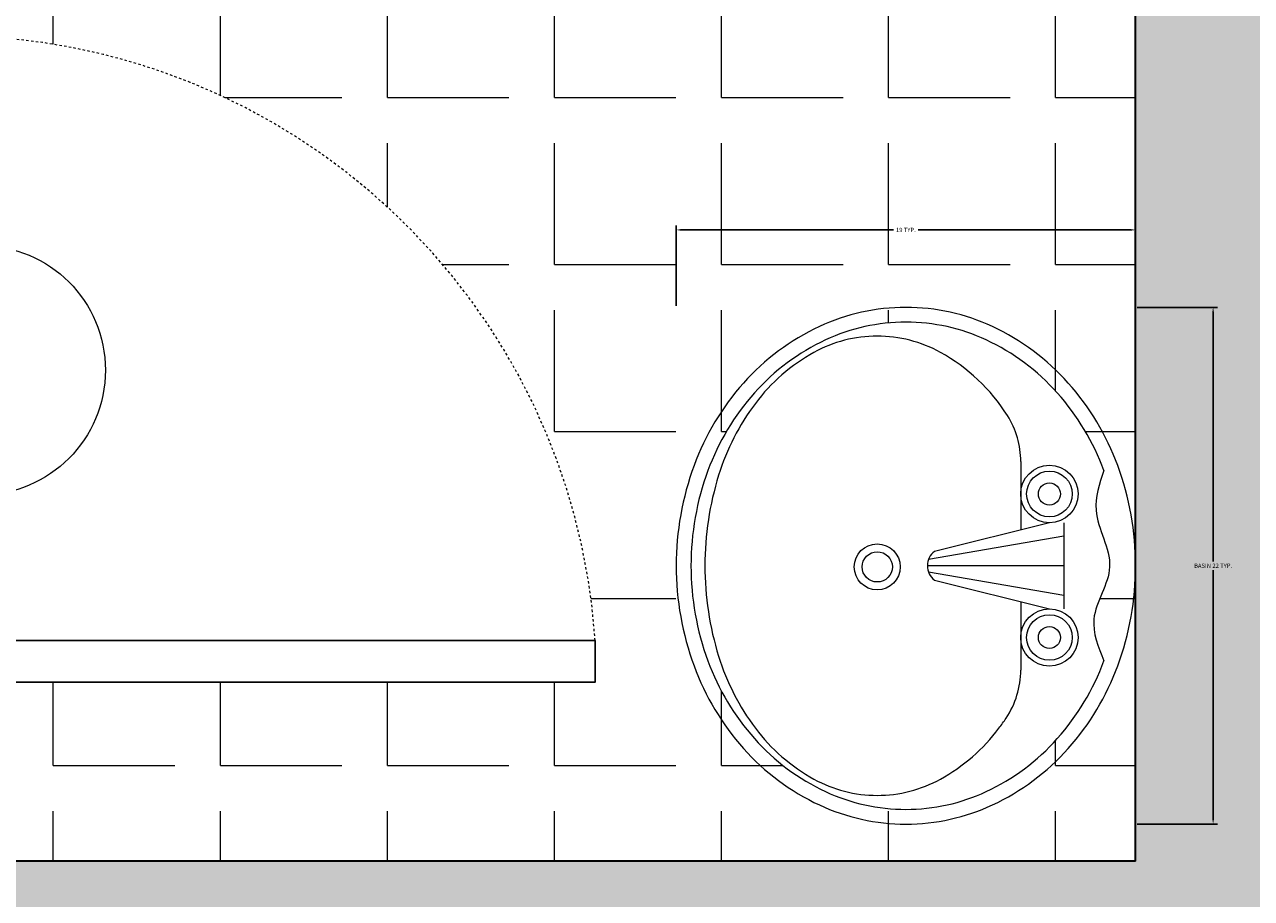
# Model space of a CAD drawing. Units: inches. Extents: x 2701 to 6846, y 811 to 2447.
# Tile 17 of 20: x 2926 to 2977, y 1370 to 1407. Entities that reach past the tile are written whole.
import ezdxf

# ---------------------------------------------------------------- set-up
doc = ezdxf.new("R2010")
doc.units = ezdxf.units.IN
doc.linetypes.add('HIDDEN4', pattern=[0.09375, 0.0625, -0.03125])
for name, color, linetype, lineweight in [('A-ANNO-DIMS', 2, 'Continuous', 18), ('A-ANNO-IDEN', 7, 'Continuous', 13), ('A-DOOR', 4, 'Continuous', 25), ('A-DOOR-SWNG', 4, 'HIDDEN4', 13), ('A-FLOR-FIXT', 7, 'Continuous', 18), ('A-FLOR-PATT', 252, 'Continuous', 13), ('A-WALL', 7, 'Continuous', 35)]:
    doc.layers.add(name, color=color, linetype=linetype, lineweight=lineweight)
doc.layers.add('A-WALL-PATT', color=18, linetype='Continuous', lineweight=13, true_color=0x000000)
doc.styles.get("Standard").update_dxf_attribs({"font": 'arial.ttf'})
doc.dimstyles.get("Standard").update_dxf_attribs({"dimtxt": 0.18, "dimasz": 0.18, "dimexe": 0.18, "dimexo": 0.0625, "dimgap": 0.09, "dimtad": 0, "dimtih": 1, "dimtoh": 1, "dimdec": 4, "dimzin": 0, "dimdsep": 46, "dimtxsty": 'Standard', "dimcen": 0.09, "dimadec": 0, "dimazin": 0, "dimtfac": 1, "dimtdec": 4, "dimtofl": 0, "dimtmove": 0, "dimatfit": 3, "dimfxl": 1, "dimtolj": 1, "dimtzin": 0, "dimarcsym": 0})

# ---------------------------------------------------------------- blocks, each defined once
blk = doc.blocks.new('A$C62EA08CE')
at = {"linetype": 'ByBlock'}
for p, q in [((0.2190750854661019, 0.3943350335612194), (0.306705085467911, 0.3943350335612194)), ((0.2328389724007138, 0.3943350335612194), (0.256592247476874, 0.2566437564746593)), ((0.2628900854706444, 0.3943350335612194), (0.2628900854706444, 0.2555161210839287)), ((0.2933077018988115, 0.3943350335612194), (0.2695802776597702, 0.256794098582759)), ((0.2190750854661019, 0.3797300335645559), (0.2482850854667049, 0.2628900335621438)), ((0.2774950854673079, 0.2628900335621438), (0.306705085467911, 0.3797300335645559)), ((0.1569030901755468, 0.3505200335639529), (0.2263775854680716, 0.3505200335639529)), ((0.2994025854659412, 0.3505200335639529), (0.3690778702966782, 0.3505200335639529))]:
    blk.add_line(p, q, dxfattribs=at)
for centre, radius in [((0.1898650854727748, 0.3797300335645559), 0.02921), ((0.1898650854727748, 0.3797300335645559), 0.02321), ((0.335915085468514, 0.3797300335645559), 0.02921), ((0.335915085468514, 0.3797300335645559), 0.02321), ((0.1898650854727748, 0.3797300335645559), 0.01121), ((0.335915085468514, 0.3797300335645559), 0.01121), ((0.2640384579517558, 0.2045255693010404), 0.023368), ((0.2640384579517558, 0.2045255693010404), 0.015368)]:
    blk.add_circle(centre, radius, dxfattribs=at)
for centre, radius, start, end in [((0.2628901093212335, 0.172201390065311), 0.2951586434963838, 90.00000458569829, 110.2131769401282), ((0.2628900616127794, 0.172201390065311), 0.2951586434963838, 69.78682305987175, 89.9999954143017), ((0.2518357941607974, 0.202225176646607), 0.2631644933429036, 110.2132031902237, 131.6335499305747), ((0.2739443767732155, 0.202225176646607), 0.2631644933429035, 48.36645006942531, 69.78679680977629), ((0.2518357941607974, 0.202225176646607), 0.2481644933429036, 110.2132031902237, 131.6335499305747), ((0.2739443767732155, 0.202225176646607), 0.2481644933429035, 48.36645006942531, 69.78679680977629), ((0.2348020259832992, 0.2213881285715615), 0.2375253048786466, 131.6335451873388, 155.0149376704166), ((0.2348020259832992, 0.2213881285715615), 0.2225253048786466, 131.6335451873388, 155.0149376704166), ((0.2909781449579896, 0.2213881285715615), 0.2225253048786464, 24.98506232958336, 48.36645481266113), ((0.2909781449579896, 0.2213881285715615), 0.2375253048786464, 24.98506232958336, 48.36645481266113), ((0.1569030901755468, 0.2628900335621438), 0.08763, 90, 122.2598079089317), ((0.3690778702966782, 0.2628900335621438), 0.08763, 56.09549019404326, 90), ((0.2106628391502454, 0.177718259532412), 0.18834914705, 122.2598079089317, 151.0887990604045), ((0.2835224813406967, 0.1355918312110589), 0.24100718245, 53.1301018541481, 56.09549019404326), ((0.3151173317910434, 0.177718259532412), 0.18834914705, 28.91120093959547, 53.1301018541481), ((0.2084237233957538, 0.23368008415855), 0.208423637924446, 155.0149182782628, 180.0000137570949), ((0.2084237233957538, 0.23368008415855), 0.1934236379244461, 155.0149182782628, 180.0000137570949), ((0.317356447545535, 0.23368008415855), 0.1934236379244455, 359.9999862429051, 24.98508172173719), ((0.317356447545535, 0.23368008415855), 0.2084236379244456, 359.9999862429051, 24.98508172173719), ((0.1622244803456851, 0.2044700335609377), 0.13301439488, 151.0887990604045, 180), ((0.2628900854706444, 0.2736666355558555), 0.018150514468869, 216.4225302188404, 323.5774697811596), ((0.3635556905883277, 0.2044700335609377), 0.13301439488, 0, 28.91120093959547), ((0.2084237233957538, 0.2336799829718075), 0.2084236379244456, 179.9999862429051, 204.9850817217372), ((0.2084237233957538, 0.2336799829718075), 0.1934236379244455, 179.9999862429051, 204.9850817217372), ((0.317356447545535, 0.2336799829718075), 0.1934236379244461, 335.0149182782628, 1.37570948859e-05), ((0.317356447545535, 0.2336799829718075), 0.208423637924446, 335.0149182782628, 1.37570948859e-05), ((0.1622244803456851, 0.2044700335609377), 0.13301439488, 180, 208.9112009395955), ((0.3635556905883277, 0.2044700335609377), 0.13301439488, 331.0887990604045, 0), ((0.2348020259832992, 0.2459719385587959), 0.2225253048786464, 204.9850623295834, 228.3664548126612), ((0.2909781449579896, 0.2459719385587959), 0.2225253048786466, 311.6335451873388, 335.0149376704167), ((0.2348020259832992, 0.2459719385587959), 0.2375253048786464, 204.9850623295834, 228.3664548126612), ((0.2106628391502454, 0.2312218075967394), 0.18834914705, 208.9112009395955, 233.1301018541481), ((0.3151173317910434, 0.2312218075967394), 0.18834914705, 306.8698981458519, 331.0887990604045), ((0.2909781449579896, 0.2459719385587959), 0.2375253048786466, 311.6335451873388, 335.0149376704167), ((0.2518357941607974, 0.2651348904837505), 0.2481644933429134, 228.3664500694253, 249.7867968097763), ((0.2422576896005921, 0.2733482359108166), 0.24100718245, 233.1301018541481, 252.7420607856108), ((0.2835224813406967, 0.2733482359108166), 0.24100718245, 287.2579392143892, 306.8698981458519), ((0.2739443767732155, 0.2651348904837505), 0.2481644933429136, 290.2132031902237, 311.6335499305747), ((0.2518357941607974, 0.2651348904837505), 0.2631644933429134, 228.3664500694253, 249.7867968097763), ((0.2739443767732155, 0.2651348904837505), 0.2631644933429136, 290.2132031902237, 311.6335499305747), ((0.2628900854706444, 0.3397629544924712), 0.31055292093, 252.7420607856108, 270), ((0.2628900854706444, 0.3397629544924712), 0.31055292093, 270, 287.2579392143892), ((0.2628901093212335, 0.2951586770577705), 0.2801586434963766, 249.7868230598717, 269.9999954143017), ((0.2628900616127794, 0.2951586770577705), 0.2801586434963765, 270.0000045856983, 290.2131769401283), ((0.2628901093212335, 0.2951586770577705), 0.2951586434963766, 249.7868230598717, 269.9999954143017), ((0.2628900616127794, 0.2951586770577705), 0.2951586434963765, 270.0000045856983, 290.2131769401283)]:
    blk.add_arc(centre, radius, start, end, dxfattribs=at)
blk.add_open_spline([(0.1660913743126002, 0.4351060694243643), (0.1795429390761559, 0.4305676737460202), (0.2123752678413389, 0.4194904420932696), (0.2631088802261481, 0.454314446693237), (0.3131553959096029, 0.4161820139975771), (0.3454695139184305, 0.4293234167515693), (0.3596887966214126, 0.4351060694243643)], degree=3, knots=[0, 0, 0, 0, 0.0411087303528805, 0.1003374234737184, 0.1559132068848227, 0.1995857666183122, 0.1995857666183122, 0.1995857666183122, 0.1995857666183122], dxfattribs=at)
blk = doc.blocks.new('DOOR-D2-30IN-PANEL-FRAME')
blk.add_lwpolyline([(-4.547e-13, 30.00000000000046), (-4.547e-13, 28.52062868157645), (4.3614931230818, 28.52062868157645), (4.3614931230818, 30.00000000000046), (-4.547e-13, 30.00000000000046)], close=True)
for points in [[(3.925343810773938, 30.00000000000046), (0.4361493129576957, 30.00000000000046)], [(4.361493123406944, 0), (4.361493123406944, 3.223968567697738), (31.40275048651847, 3.22396856790101), (31.40275048651847, 1.479371318667745), (1.623448e-10, 1.479371318424), (1.623448e-10, 0)], [(1.623448e-10, 0), (4.361493123406944, 0)], [(3.925343810773938, 0), (0.4361493129576957, 0)]]:
    blk.add_lwpolyline(points)
blk = doc.blocks.new('*D39')
at = {"layer": 'A-ANNO-DIMS', "color": 0, "lineweight": -2, "transparency": 16777216}
for p, q in [((2972.033891037219, 1395.209040201173), (2975.392713579943, 1395.209040201173)), ((2975.212713579943, 1395.029040201173), (2975.212713579943, 1384.58770130251)), ((2975.212713579943, 1373.780223249686), (2975.212713579943, 1384.221562148349)), ((2972.033891037219, 1373.600223249686), (2975.392713579943, 1373.600223249686))]:
    blk.add_line(p, q, dxfattribs=at)
at = {"layer": 'A-ANNO-DIMS', "color": 0, "transparency": 16777216}
for points in [[(2975.182713579943, 1395.029040201173), (2975.242713579943, 1395.029040201173), (2975.212713579943, 1395.209040201173)], [(2975.182713579943, 1373.780223249686), (2975.242713579943, 1373.780223249686), (2975.212713579943, 1373.600223249686)]]:
    blk.add_solid(points, dxfattribs=at)
at = {"layer": 'Defpoints', "color": 0, "transparency": 16777216}
for p in [(2971.971391037218, 1395.209040201173), (2971.971391037218, 1373.600223249686), (2975.212713579943, 1373.600223249686)]:
    blk.add_point(p, dxfattribs=at)
at = {"layer": 'A-ANNO-DIMS', "color": 0, "transparency": 16777216, "insert": (2975.212713579943, 1384.404631725428), "char_height": 0.18, "attachment_point": 5}
blk.add_mtext('\\A1;BASIN 22 TYP.', dxfattribs=at)
blk = doc.blocks.new('*D40')
at = {"layer": 'A-ANNO-DIMS', "color": 0, "lineweight": -2, "transparency": 16777216}
for p, q in [((2952.763554280548, 1395.271540201173), (2952.763554280548, 1398.630362743896)), ((2952.943554280548, 1398.450362743896), (2961.847854650697, 1398.450362743896)), ((2971.791391037218, 1398.450362743896), (2962.887090667068, 1398.450362743896)), ((2971.971391037218, 1395.271540201173), (2971.971391037218, 1398.630362743896))]:
    blk.add_line(p, q, dxfattribs=at)
at = {"layer": 'A-ANNO-DIMS', "color": 0, "transparency": 16777216}
for points in [[(2952.943554280548, 1398.480362743896), (2952.943554280548, 1398.420362743896), (2952.763554280548, 1398.450362743896)], [(2971.791391037218, 1398.480362743896), (2971.791391037218, 1398.420362743896), (2971.971391037218, 1398.450362743896)]]:
    blk.add_solid(points, dxfattribs=at)
at = {"layer": 'Defpoints', "color": 0, "transparency": 16777216}
for p in [(2971.971391037218, 1398.450362743896), (2952.763554280548, 1395.209040201173), (2971.971391037218, 1395.209040201173)]:
    blk.add_point(p, dxfattribs=at)
at = {"layer": 'A-ANNO-DIMS', "color": 0, "transparency": 16777216, "insert": (2962.367472658883, 1398.450362743896), "char_height": 0.18, "attachment_point": 5}
blk.add_mtext('\\A1;19 TYP.', dxfattribs=at)

msp = doc.modelspace()

# ---------------------------------------------------------------- hatches: boundary and pattern name
at = {"layer": 'A-FLOR-PATT'}
h = msp.add_hatch(dxfattribs=at)
h.set_pattern_fill('ANGLE', color=256)
h.set_pattern_definition([(0, (0, 0), (0, 6.985), [5.08, -1.905]), (90, (0, 0), (-6.985, 4e-16), [5.08, -1.905])])
h.paths.add_polyline_path([(2841.812531618507, 1296.510714093028, -0.1094531397224823), (2842.614165366529, 1300.128842847245, -0.1023747835315324), (2844.977063233859, 1303.301704019213, -0.0937428406070795), (2848.425874088265, 1305.367635711971, -0.0624630522953803), (2851.366818664733, 1306.050044742079), (2785.971391037217, 1306.050044742079), (2785.971391037217, 1258.050044742079), (2827.971391037217, 1258.050044742079), (2827.971391037217, 1256.411537864998), (2829.450762355621, 1256.411537864998, -0.3948265708167148), (2854.747422469505, 1283.452795228435), (2856.49201971855, 1283.452795228435), (2856.49201971876, 1256.411537865324), (2857.971391037219, 1256.411537865324), (2857.971391037219, 1258.05004474208), (2863.971391037218, 1258.050044742079), (2863.971391037217, 1306.050044742079), (2853.867060923166, 1306.050044742079, -0.0624630504647152), (2856.808005416599, 1305.367635742541, -0.0937428427235612), (2860.256816355725, 1303.301704017657, -0.1023747714125829), (2862.619714024758, 1300.128843269809, -0.1094531521575188), (2863.421347969692, 1296.510714138194, -0.109453153989093), (2862.619714017641, 1292.892584946142, -0.1023747709767553), (2860.256816355757, 1289.719724213534, -0.093738257087872), (2856.808189965141, 1287.653860434733, -0.0884250558281599), (2852.616939784454, 1286.906795737127, -0.0884250554332989), (2848.425689622791, 1287.653860434813, -0.0937382570330623), (2844.977063234018, 1289.719724212192, -0.1023747824199799), (2842.614165384649, 1292.892585345091, -0.1094531396555831)])
h.paths.add_polyline_path([(2805.214857085719, 1273.877134568363, -0.141745245190178), (2808.318689175414, 1271.772621468736, -0.1849834247598648), (2809.773740825251, 1267.974277286972, -0.1849834247688995), (2808.318689175285, 1264.175933105053, -0.141745244968364), (2805.214857091107, 1262.071420007333, -0.1522440861962393), (2799.994488829542, 1261.79557176336, -0.0256138964539793), (2799.368711507224, 1261.94541476925), (2794.365115778627, 1263.418098821323), (2794.36467071784, 1263.405353947873, -0.1112416791490392), (2793.99312620013, 1261.915170284834, -0.0338893268367682), (2793.114424873909, 1260.113565580275, -0.286745385218), (2792.375651823606, 1259.651928944151), (2787.580775843661, 1259.651928944133, -0.4142135623681101), (2787.152671505053, 1260.080033282747), (2787.152671505153, 1267.974277286972), (2787.152671505053, 1275.868521290948, -0.4142135623730951), (2787.580775843668, 1276.296625629562), (2792.375651823623, 1276.296625629544, -0.2867453846084762), (2793.114424873105, 1275.834988995069, -0.0338893268640583), (2793.99312620013, 1274.033384289111, -0.1051042356073151), (2794.361711671137, 1272.627936636842), (2794.365115778619, 1272.530455752619), (2799.368711507498, 1274.003139804786, -0.0256138965941945), (2799.994488833287, 1274.152982811292, -0.1522440859162748)], flags=16)
h.paths.add_polyline_path([(2804.681063364808, 1272.339952816459, -0.1449445299175104), (2807.087654609562, 1270.708506585421, -0.0358001151589041), (2807.447023191777, 1270.252713401882, -0.1332846890906797), (2807.893417732773, 1268.607871708063), (2807.893417732813, 1267.974277286972), (2807.893417732773, 1267.340682865632, -0.1332846888970446), (2807.447023193029, 1265.695841173949, -0.0358001152638917), (2807.087654609923, 1265.240047988954, -0.1449445297267833), (2804.681063368992, 1263.608601758809, -0.1554037438169349), (2800.343099481134, 1263.385728797012, -0.3645106918446579), (2796.485382154562, 1267.974277286972, -0.3645106920174053), (2800.343099483932, 1272.562825777418, -0.1554037435534987)], flags=0)
h.paths.add_polyline_path([(2800.015880108981, 1268.901471623875, 0.1692977046764319), (2799.131174998024, 1268.11576383613, 0.0766670309700064), (2799.100009657075, 1267.974277286936, 0.0766670313951798), (2799.13117499834, 1267.832790736999, 0.1692977045836763), (2800.015880108981, 1267.04708294982, 0.3052192884941762), (2800.365297210358, 1267.156497374013, 0.1695347489604994), (2800.650786991011, 1267.974277286972, 0.1695347391656343), (2800.365297241503, 1268.792057160761, 0.3052193300480048)], flags=0)
h.paths.add_polyline_path([(2971.971391037218, 1456.050044742079), (2923.971391037218, 1456.050044742079), (2923.971391037218, 1408.050044742079), (2922.332884160136, 1408.050044742079), (2922.332884160136, 1406.570673423676, -0.394826570816717), (2949.374141523573, 1381.274013309792), (2949.374141523573, 1379.529416060747), (2922.332884160461, 1379.529416060537), (2922.332884160461, 1378.050044742079), (2923.971391037218, 1378.050044742079), (2923.971391037217, 1372.050044742079), (2971.971391037217, 1372.050044742079)])
h.paths.add_polyline_path([(2939.8177624336, 1436.526417411941, -0.1417452451905352), (2937.713249333971, 1433.422585322236, -0.1849834247599418), (2933.914905152205, 1431.967533672398, -0.1849834247691276), (2930.116560970283, 1433.422585322367, -0.1417452449676952), (2928.01204787257, 1436.526417406529, -0.1522440861964963), (2927.736199628592, 1441.746785668103, -0.0256138964540868), (2927.886042634483, 1442.372562990423), (2929.358726686557, 1447.376158719022), (2929.345981813088, 1447.376603779809, -0.1112416791473441), (2927.855798150072, 1447.748148297517, -0.0338893268369074), (2926.054193445506, 1448.626849623741, -0.2867453852169366), (2925.592556809384, 1449.365622674043), (2925.592556809366, 1454.160498653989, -0.4142135623681173), (2926.020661147981, 1454.588602992596), (2933.914905152205, 1454.588602992496), (2941.809149156182, 1454.588602992596, -0.4142072303161659), (2942.237253494696, 1454.160507909187), (2942.237253494777, 1449.365622674043, -0.2867453846243844), (2941.775616860276, 1448.626849624529, -0.0338893268635044), (2939.974012154347, 1447.74814829752, -0.1051042356087532), (2938.568564502058, 1447.379562826511), (2938.471083617852, 1447.37615871903), (2939.943767670019, 1442.372562990154, -0.0256138965942444), (2940.093610676525, 1441.746785664364, -0.152244085915992)], flags=16)
h.paths.add_polyline_path([(2938.280580681695, 1437.060211132847, -0.1449445299182329), (2936.649134450649, 1434.653619888082, -0.0358001151583613), (2936.193341267117, 1434.294251305872, -0.1332846890907526), (2934.548499573297, 1433.847856764876), (2933.914905152205, 1433.847856764836), (2933.281310730865, 1433.847856764876, -0.1332846888976268), (2931.636469039176, 1434.294251304624, -0.0358001152630847), (2931.180675854191, 1434.653619887722, -0.14494452972667), (2929.549229624045, 1437.06021112865, -0.1554037438170702), (2929.326356662246, 1441.398175016512, -0.3645106918448713), (2933.914905152205, 1445.255892343087, -0.3645106920173691), (2938.503453642651, 1441.398175013717, -0.1554037435532691)], flags=0)
h.paths.add_polyline_path([(2969.158462562638, 1392.044508285666, -0.0937428443921736), (2971.224394311477, 1388.595697278927, -0.0884209696484748), (2971.971391037217, 1384.404631716083, -0.0884209680179829), (2971.224394332037, 1380.213566228077, -0.0937428458331012), (2969.158462561081, 1376.764755163806, -0.1023747798731684), (2965.985601516888, 1374.401857356678, -0.1094531425013952), (2962.367472681615, 1373.600223549837, -0.1094531553411192), (2958.74934344807, 1374.401857521223, -0.102374769792102), (2955.576482756955, 1376.764755163771, -0.0937382570879047), (2953.510618978154, 1380.213381554388, -0.0884250558281564), (2952.763554280548, 1384.404631735075, -0.0884250554336261), (2953.510618978239, 1388.595881896752, -0.0937382570324601), (2955.576482755607, 1392.044508285504, -0.1023747638736991), (2958.749343238892, 1394.40740583216, -0.10945316082308), (2962.367472636449, 1395.209039901022, -0.1094531494878097), (2965.985601690358, 1394.407406013345, -0.102374774975509)], flags=0)
edge = h.paths.add_edge_path(flags=16)
edge.add_arc((2961.074722408913, 1384.858947505427), 10.19921062335061, 20.21320321302568, 41.63359467655653, ccw=False)
edge.add_spline(control_points=[(2970.645798607602, 1388.382922212802), (2970.45927694694, 1387.830081875375), (2970.004018351208, 1386.480719475378), (2971.435235818619, 1384.395639569603), (2969.86804662324, 1382.338798369057), (2970.408139739579, 1381.010733700175), (2970.645798607602, 1380.426341238356)], knot_values=[0, 0, 0, 0, 0.0411087303528805, 0.1003374234737184, 0.1559132068848227, 0.1995857666183122, 0.1995857666183122, 0.1995857666183122, 0.1995857666183122], degree=3, periodic=0)
edge.add_arc((2961.074722408954, 1383.950315945844), 10.19921062335061, 318.3664053106646, 339.7867967863075, ccw=False)
edge.add_arc((2961.862292702369, 1383.250252100635), 9.145476143303874, 294.98529005245234, 318.3664053112933, ccw=False)
edge.add_arc((2962.367474738348, 1382.166141072693), 7.949438681384353, 269.9999862429006, 294.9853451035073, ccw=False)
edge.add_arc((2962.367470579714, 1382.166141072693), 7.949438681384465, 245.0146528606722, 270.00001621636034, ccw=False)
edge.add_arc((2962.872652615592, 1383.250252100682), 9.145476143303885, 221.633594689284, 245.0147081786685, ccw=False)
edge.add_arc((2963.660222908995, 1383.950315945905), 10.19921062335051, 200.2129623510071, 221.6335946899624, ccw=False)
edge.add_arc((2964.894158186733, 1384.404632705954), 11.5141250647146, 180.0000045856949, 200.2129623497761, ccw=False)
edge.add_arc((2964.894158186734, 1384.404630744956), 11.51412506471477, 159.7870376490639, 179.999994827515, ccw=False)
edge.add_arc((2963.660222908922, 1384.858947504804), 10.19921062335051, 138.3664053200289, 159.7870376464858, ccw=False)
edge.add_arc((2962.872652615694, 1385.559011350224), 9.145476143303881, 114.9852895697228, 138.3664053235114, ccw=False)
edge.add_arc((2962.367470579715, 1386.643122378167), 7.949438681384341, 89.99998624290072, 114.9853445481478, ccw=False)
edge.add_arc((2962.367474738348, 1386.643122378167), 7.949438681384461, 65.01465414332972, 90.00001621635698, ccw=False)
edge.add_arc((2961.862292702924, 1385.559011349966), 9.145476143303876, 41.63359468007258, 65.01470929671348, ccw=False)
h.paths.add_polyline_path([(2963.809881193461, 1393.327235568244, -0.1264579126559968), (2966.613496696745, 1390.682864813822, -0.1416969839114421), (2967.169431848072, 1388.76054773013), (2967.169431848171, 1387.405856218539, -1), (2969.570411442753, 1387.40585621857, -0.4142135626407067), (2968.369921644365, 1386.205366421279), (2963.567962456663, 1385.004876624353, 0.146217798515541), (2963.311249278865, 1384.663463983469), (2968.97016654397, 1385.639690083447), (2968.97016654397, 1383.154510596366), (2963.317428127216, 1384.129674263443, 0.1403115373898127), (2963.56796245605, 1383.804386826958), (2968.369921645561, 1382.603897029581, -0.4142135623489124), (2969.570411442753, 1381.403407232289, -1), (2967.169431848171, 1381.403407232289), (2967.169431848072, 1380.040463554169, -0.1490250791000606), (2966.557068512987, 1378.031526062613, -0.0127594246128423), (2966.264512020975, 1377.619349736432, -0.1063032105074506), (2963.809880694587, 1375.482028786924, -0.1268223860120219), (2961.166982861567, 1374.800713347196, -0.12682239841106), (2958.52408452876, 1375.482027883284, -0.1063031789236789), (2956.069454414507, 1377.619348785205, -0.0857220920089208), (2954.537253221299, 1380.622635309784, -0.0753510219692474), (2953.964044077883, 1384.404631725429, -0.0753510220208753), (2954.537253222076, 1388.186628143578, -0.0857220919249397), (2956.069454414099, 1391.189914665108, -0.1063031717113424), (2958.5240850283, 1393.327234664099, -0.1268223860250843), (2961.166982861567, 1394.008550103962, -0.1268223983642548)], flags=0)
h.paths.add_polyline_path([(2934.842099489099, 1441.725394388693, 0.1692977046741335), (2934.056391701355, 1442.610099499628, 0.0766670309649834), (2933.91490515217, 1442.641264840574, 0.0766670314095982), (2933.773418602207, 1442.610099499295, 0.1692977045780331), (2932.987710815057, 1441.72539438868, 0.305219290057435), (2933.097125240708, 1441.375977286128, 0.169534748594888), (2933.914905152205, 1441.090487506638, 0.1695347390414705), (2934.732685025499, 1441.375977255749, 0.3052193305973386)], flags=0)
h.paths.add_polyline_path([(2969.323819906164, 1387.40585621857, -1), (2967.416023384759, 1387.40585621857, -1)], flags=0)
h.paths.add_polyline_path([(2968.830636832988, 1387.40585621857, -1), (2967.909206457936, 1387.40585621857, -1)], flags=0)
h.paths.add_polyline_path([(2962.129657139981, 1384.357435236314, -1), (2960.208873464314, 1384.357435236314, -1)], flags=0)
h.paths.add_polyline_path([(2961.800868424529, 1384.357435236314, -1), (2960.537662179766, 1384.357435236314, -1)], flags=0)
h.paths.add_polyline_path([(2969.323819906164, 1381.403407232289, -1), (2967.416023384759, 1381.403407232289, -1)], flags=0)
h.paths.add_polyline_path([(2968.830636832988, 1381.403407232289, -1), (2967.909206457936, 1381.403407232289, -1)], flags=0)
h.paths.add_polyline_path([(3085.971391037217, 1306.050044742079), (3001.971391037217, 1306.050044742079), (3001.971391037217, 1300.050044742079), (3000.332884160462, 1300.050044742079), (3000.332884160462, 1298.570673423621), (3027.374141523574, 1298.570673423411), (3027.374141523574, 1296.826076174374, -0.3948265708167921), (3000.332884160137, 1271.529416060482), (3000.332884160137, 1270.050044742079), (3001.971391037216, 1270.050044742079), (3001.971391037217, 1258.050044742079), (3085.971391037217, 1258.050044742079)])
h.paths.add_polyline_path([(3033.332715044416, 1274.444953022308, -0.1023747723857111), (3035.695612729331, 1271.272092240373, -0.1094531510467398), (3036.49724665838, 1267.653963142847, -0.109453129065687), (3035.695613062762, 1264.035834715682, -0.102374792813879), (3033.332715044451, 1260.862973218194, -0.0937428491083937), (3029.883903848349, 1258.797041398739, -0.0884209654955001), (3025.692838473141, 1258.05004474208, -0.0884209669723455), (3021.501773032378, 1258.797041429867, -0.093742846952782), (3018.052961922706, 1260.862973216846, -0.1023747779170817), (3015.690064146835, 1264.035834192024, -0.1094531447948728), (3014.888430307195, 1267.653963097683, -0.1094531229044609), (3015.690063814699, 1271.272091335764, -0.1023747982671114), (3018.052961922546, 1274.444953023867, -0.0937382570344717), (3021.501588311451, 1276.510816801145, -0.0884250558280669), (3025.692838492134, 1277.25788149875, -0.0884250554332868), (3029.884088653796, 1276.510816801064, -0.0937382570874262)], flags=0)
edge = h.paths.add_edge_path(flags=16)
edge.add_arc((3026.847218107582, 1267.148783163603), 9.145476143303444, 24.985288685417686, 48.36640531129461, ccw=False)
edge.add_arc((3027.931329135525, 1267.653965199581), 7.949438681383711, -1.3757099395661498e-05, 24.98534353079839, ccw=False)
edge.add_arc((3027.931329135525, 1267.653961040948), 7.949438681383458, -24.98534255728248, 1.6216352207720774e-05, ccw=False)
edge.add_arc((3026.847218107536, 1268.159143076827), 9.145476143303622, 311.6335946892918, 335.0147121614734, ccw=False)
edge.add_arc((3026.147154262487, 1268.946713370386), 10.19921062335084, 290.21320321300624, 311.633594688656, ccw=False)
edge.add_spline(control_points=[(3029.671128969861, 1259.375637171695), (3029.086736508042, 1259.613296039718), (3027.758671839159, 1260.153389156057), (3025.701830638613, 1258.586199960678), (3023.616750732838, 1260.01741742809), (3022.267388332841, 1259.562158832357), (3021.714547995414, 1259.375637171695)], knot_values=[0, 0, 0, 0, 0.0436725597334895, 0.0992483431445938, 0.1584770362654316, 0.1995857666183122, 0.1995857666183122, 0.1995857666183122, 0.1995857666183122], degree=3, periodic=0)
edge.add_arc((3025.238522703413, 1268.946713370155), 10.19921062335076, 228.3664053199745, 249.78679678323948, ccw=False)
edge.add_arc((3024.538458857992, 1268.159143076927), 9.145476143303437, 204.9852869984493, 228.3664053234469, ccw=False)
edge.add_arc((3023.45434783005, 1267.65396104095), 7.949438681383719, 179.9999862429023, 204.9853415900221, ccw=False)
edge.add_arc((3023.454347830049, 1267.653965199583), 7.949438681383464, 155.0146544340279, 180.0000162163587, ccw=False)
edge.add_arc((3024.538458858251, 1267.148783164158), 9.14547614330361, 131.6335946800857, 155.0147095493943, ccw=False)
edge.add_arc((3025.238522702964, 1266.361212870303), 10.19921062335009, 110.2129623509966, 131.6335946778856, ccw=False)
edge.add_arc((3025.692839463013, 1265.127277592565), 11.51412506471423, 90.00000458569599, 110.2129623497689, ccw=False)
edge.add_arc((3025.692837502014, 1265.127277592564), 11.51412506471427, 69.78703764905441, 89.99999482750928, ccw=False)
edge.add_arc((3026.147154262372, 1266.361212870188), 10.19921062335108, 48.3664053106545, 69.78703764952758, ccw=False)
h.paths.add_polyline_path([(3032.478121424384, 1273.951981363762, -0.1063031716151077), (3034.615441420988, 1271.497350751304, -0.1268223860413822), (3035.296756861021, 1268.85445291773, -0.1268223983836015), (3034.615442325363, 1266.211554585404, -0.1063032176830601), (3032.478120473694, 1263.756923759752, -0.012759424397259), (3032.06594390682, 1263.464367621596, -0.1490250698458729), (3030.057006653981, 1262.852003931225), (3028.694062975896, 1262.852003931126, -0.4142135623806731), (3029.894552773218, 1261.651514133835, -1), (3027.493573178635, 1261.651514133737), (3026.293083381258, 1266.453473323247, 0.1403115373895235), (3025.967795944775, 1266.704007652081), (3026.94295961185, 1261.051269235327), (3024.457780124769, 1261.051269235327), (3025.434006224748, 1266.710186500432, 0.1462177985154153), (3025.092593583864, 1266.453473322634), (3023.892103786938, 1261.651514134932, -1.000000100073327), (3021.491124192355, 1261.651514133836, -0.4142135623731147), (3022.691613989647, 1262.852003931127), (3021.336922478021, 1262.852003931226, -0.1416970043012063), (3019.41460486282, 1263.407938240376, -0.1264579123471447), (3016.770235543815, 1266.211555085013, -0.1268223859959933), (3016.088920104255, 1268.854452917731, -0.1268223983918172), (3016.770234640404, 1271.497351250108, -0.1063031789240722), (3018.907555542179, 1273.951981364503, -0.0857220919129331), (3021.910842063079, 1275.484182556737, -0.0753510220530541), (3025.692838482788, 1276.057391701414, -0.075351022008823), (3029.474834900351, 1275.484182557402, -0.0857220920013936)], flags=0)
h.paths.add_polyline_path([(3072.364663406136, 1280.00178826655, -0.1849834247682267), (3076.163007588042, 1281.456839916512, -0.1849834247587431), (3079.961351769785, 1280.001788266685, -0.1417452451922909), (3082.065864869442, 1276.897956176945, -0.1522440859149591), (3082.341713112365, 1271.677587924556, -0.0256138965949624), (3082.191870105855, 1271.051810598748), (3080.719186053688, 1266.048214869872), (3080.816666937894, 1266.04481076239, -0.1051042356089094), (3082.222114590184, 1265.676225291381, -0.0338893268638024), (3084.023719296129, 1264.797523964363, -0.2867453846178035), (3084.485355930614, 1264.058750914859), (3084.485355930532, 1259.26388419012, -0.4142198944533688), (3084.057251592018, 1258.835770596306), (3076.163007588042, 1258.835770596406), (3068.268763583817, 1258.835770596306, -0.4142135623730951), (3067.840659245203, 1259.26387493492), (3067.84065924522, 1264.058750914876, -0.2867453852273427), (3068.302295881383, 1264.797523965184, -0.0338893268359893), (3070.103900585901, 1265.676225291382, -0.1051042356607345), (3071.509348238908, 1266.044810762424), (3071.606829122393, 1266.04821486988), (3070.134145070319, 1271.051810598479, -0.0256138964541135), (3069.984302064428, 1271.6775879208, -0.1522440861962023), (3070.260150308403, 1276.897956182364, -0.1417452449689107)], flags=16)
h.paths.add_polyline_path([(3073.428778290028, 1278.770753701179, -0.0358001152649927), (3073.884571475038, 1279.130122284293, -0.1332846888953009), (3075.529413166701, 1279.576516824026), (3076.163007588042, 1279.576516824066), (3076.796602009133, 1279.576516824026, -0.1332846890885353), (3078.441443702929, 1279.130122283046, -0.0358001151610664), (3078.897236886497, 1278.77075370081, -0.1449445299169966), (3080.528683117528, 1276.364162456064, -0.1554037435538929), (3080.751556078487, 1272.026198575177, -0.3645106920168784), (3076.163007588042, 1268.168481245816, -0.3645106918444272), (3071.574459098083, 1272.026198572385, -0.1554037438173037), (3071.797332059881, 1276.364162460253, -0.1449445297265802)], flags=0)
h.paths.add_polyline_path([(3026.700426809735, 1268.85217047715, -1), (3024.77964313407, 1268.85217047715, -1)], flags=0)
h.paths.add_polyline_path([(3026.371638094284, 1268.85217047715, -1), (3025.108431849521, 1268.85217047715, -1)], flags=0)
h.paths.add_polyline_path([(3075.268500788244, 1271.624470471877, 0.1576769337924287), (3076.021521038093, 1270.814274089584, 0.0766670314188588), (3076.163007588078, 1270.783108748328, 0.0766670308737057), (3076.3044941371, 1270.814274089222, 0.1576769338966524), (3077.057514387587, 1271.624470471873, 0.3746263233786361), (3076.980787467475, 1272.048396328269, 0.1695347405768383), (3076.163007588042, 1272.333886082264, 0.1695347491173554), (3075.345227674456, 1272.04839630111, 0.3746262855823952)], flags=0)
h.paths.add_polyline_path([(3029.64796123663, 1261.651514133835, -1), (3027.740164715224, 1261.651514133835, -1)], flags=0)
h.paths.add_polyline_path([(3029.154778163453, 1261.651514133835, -1), (3028.233347788401, 1261.651514133835, -1)], flags=0)
h.paths.add_polyline_path([(3023.645512250349, 1261.651514133836, -1), (3021.737715728944, 1261.651514133836, -1)], flags=0)
h.paths.add_polyline_path([(3023.152329177172, 1261.651514133836, -1), (3022.23089880212, 1261.651514133836, -1)], flags=0)
h.paths.add_polyline_path([(2810.572659831725, 1281.221625132062), (2833.310943898055, 1281.221625132062), (2833.310943898055, 1296.429027198873), (2810.572659831725, 1296.429027198873)], flags=24)
h.paths.add_polyline_path([(2937.545180300932, 1410.244315705433), (2960.208482391776, 1410.244315705433), (2960.208482391776, 1425.451717772244), (2937.545180300932, 1425.451717772244)], flags=24)
h.paths.add_polyline_path([(3043.227580059905, 1273.098575462184), (3065.890882150748, 1273.098575462184), (3065.890882150748, 1288.305977528995), (3043.227580059905, 1288.305977528995)], flags=24)
at = {"layer": 'A-WALL-PATT'}
h = msp.add_hatch(color=256, dxfattribs=at)
h.dxf.hatch_style = 1
h.paths.add_polyline_path([(3085.971391037218, 1456.050044742079), (3085.971391037217, 1348.050044742079), (3091.971391037218, 1348.050044742079), (3091.971391037218, 1360.050044742079), (3091.971391037218, 1462.050044742079), (2960.086244240269, 1462.050044742079), (2960.086244240269, 1456.050044742079), (2971.971391037218, 1456.050044742079), (2971.971391037217, 1372.050044742079), (2923.971391037217, 1372.050044742079), (2923.971391037218, 1378.050044742079), (2917.971391037217, 1378.050044742079), (2917.971391037217, 1351.050044742079), (2923.971391037218, 1351.050044742079), (2923.971391037217, 1366.050044742079), (2971.971391037218, 1366.050044742079), (2971.971391037218, 1351.05004474208), (2976.76903347243, 1351.05004474208), (2977.971391037218, 1351.050044742079), (2977.971391037218, 1456.050044742079)])
h.paths.add_polyline_path([(2779.971391037218, 1462.050044742079), (2779.971391037218, 1342.05004474208), (2785.971391037217, 1342.05004474208), (2785.971391037218, 1456.050044742079), (2917.971391037218, 1456.050044742079), (2917.971391037217, 1408.050044742079), (2922.332884160136, 1408.050044742079), (2923.971391037218, 1408.050044742079), (2923.971391037218, 1456.050044742079), (2937.086244240269, 1456.050044742079), (2937.086244240269, 1462.050044742079)])
h.paths.add_polyline_path([(2779.971391037217, 1306.050044742079), (2779.971391037217, 1294.241199564278), (2785.971391037217, 1294.241199564278), (2785.971391037217, 1306.050044742079), (2851.366818664733, 1306.050044742079, -0.0258153414615714), (2852.616939803445, 1306.114632493797, -0.0258153410699148), (2853.867060923166, 1306.050044742079), (2863.971391037217, 1306.050044742079), (2863.971391037218, 1258.050044742079), (2857.971391037219, 1258.05004474208), (2857.971391037218, 1252.050044742079), (2878.971391037217, 1252.050044742079), (2878.971391037217, 1258.050044742079), (2869.971391037218, 1258.050044742079), (2869.971391037217, 1306.050044742079), (2923.971391037217, 1306.050044742079), (2923.971391037218, 1318.050044742079), (2919.173748601648, 1318.050044742079), (2917.971391037216, 1318.050044742079), (2917.971391037216, 1312.050044742079), (2785.971391037217, 1312.050044742079), (2785.971391037217, 1318.050044742079), (2779.971391037217, 1318.050044742079)])
h.paths.add_polyline_path([(2785.971391037218, 1252.050044742079), (2827.971391037217, 1252.050044742079), (2827.971391037217, 1256.411537864998), (2827.971391037217, 1258.050044742079), (2785.971391037217, 1258.050044742079), (2785.971391037217, 1271.241199564278), (2779.971391037218, 1271.241199564278), (2779.971391037218, 1174.050044742079), (2785.971391037217, 1174.050044742079)])
h.paths.add_polyline_path([(2779.971391037218, 1030.050044742079), (2869.971391037218, 1030.050044742079), (2869.971391037218, 1036.050044742079), (2785.971391037218, 1036.050044742079), (2785.971391037217, 1126.050044742079), (2917.971391037217, 1126.050044742079), (2917.971391037216, 1120.050044742079), (2923.971391037218, 1120.050044742078), (2923.971391037218, 1258.050044742079), (2911.971391037217, 1258.050044742079), (2911.971391037217, 1253.252402306509), (2911.971391037218, 1252.050044742079), (2917.971391037218, 1252.050044742079), (2917.971391037217, 1132.050044742078), (2785.971391037217, 1132.050044742079), (2785.971391037217, 1144.050044742079), (2779.971391037218, 1144.050044742079)])
h.paths.add_polyline_path([(2935.971391037218, 1030.050044742079), (2935.971391037218, 1033.050044742079), (2935.971391037217, 1036.050044742079), (2923.971391037218, 1036.050044742079), (2923.971391037218, 1087.050044742077), (2919.173748602005, 1087.050044742077), (2917.971391037216, 1087.050044742079), (2917.971391037218, 1036.050044742079), (2893.971391037218, 1036.050044742079), (2893.971391037218, 1030.050044742079)])
h.paths.add_polyline_path([(2971.971391037218, 1036.050044742079), (2971.971391037218, 1030.050044742079), (3091.971391037218, 1030.050044742079), (3091.971391037218, 1060.050044742079), (3085.971391037217, 1060.050044742079), (3085.971391037217, 1036.050044742079)])
h.paths.add_polyline_path([(3085.971391037217, 1084.050044742079), (3091.971391037217, 1084.050044742079), (3091.971391037217, 1096.050044742079), (3091.971391037217, 1268.891476913671), (3085.971391037217, 1268.891476913671), (3085.971391037217, 1258.050044742079), (3001.971391037217, 1258.050044742079), (3001.971391037216, 1270.050044742079), (2995.971391037217, 1270.050044742079), (2995.971391037217, 1252.050044742079), (3085.971391037217, 1252.050044742079)])
h.paths.add_polyline_path([(3085.971391037217, 1306.050044742078), (3085.971391037217, 1291.891476913671), (3091.971391037218, 1291.891476913671), (3091.971391037218, 1318.050044742079), (3085.971391037217, 1318.050044742079), (3085.971391037217, 1312.050044742079), (2977.971391037218, 1312.050044742079), (2977.971391037217, 1318.050044742079), (2971.971391037218, 1318.050044742079), (2971.971391037218, 1306.050044742079), (2995.971391037217, 1306.050044742079), (2995.971391037217, 1300.050044742079), (3000.332884160462, 1300.050044742079), (3001.971391037217, 1300.050044742079), (3001.971391037217, 1306.050044742079)])

# ---------------------------------------------------------------- linework, layer by layer
at = {"layer": 'A-ANNO-IDEN'}
msp.add_circle((2923.681908773834, 1392.582962616004), 5.217112562990953, dxfattribs=at)
at = {"layer": 'A-DOOR-SWNG'}
msp.add_arc((2922.332884160461, 1379.469257534729), 27.10141588894677, 3.818304866585595, 90, dxfattribs=at)
at = {"layer": 'A-WALL'}
for p, q in [((2971.971391037217, 1372.050044742079), (2971.971391037218, 1456.050044742079)), ((2971.971391037218, 1372.050044742079), (2923.971391037217, 1372.050044742079))]:
    msp.add_line(p, q, dxfattribs=at)

# ---------------------------------------------------------------- block references
at = {"layer": 'A-DOOR'}
msp.add_blockref('DOOR-D2-30IN-PANEL-FRAME', (2917.971391037054, 1378.050044742079), dxfattribs=at)
at = {"layer": 'A-FLOR-FIXT', "xscale": 41.09858943139644, "yscale": 41.09858943139644, "zscale": 41.09858943139644, "rotation": 270}
msp.add_blockref('A$C62EA08CE', (2952.763552901222, 1395.209043413772), dxfattribs=at)

# ---------------------------------------------------------------- dimensions: what is measured, and where the dimension line sits
at = {"layer": 'A-ANNO-DIMS'}
dim = msp.add_linear_dim(base=(2971.971391037218, 1398.450362743896), p1=(2952.763554280548, 1395.209040201173), p2=(2971.971391037218, 1395.209040201173), text='<> TYP.', dimstyle='Standard', override={"dimdec": 0, "dimlfac": 1, "dimrnd": 0, "dimzin": 0, "dimdsep": 46, "dimlunit": 2}, dxfattribs=at)
dim.commit()
dim.dimension.update_dxf_attribs({"geometry": '*D40', "text_midpoint": (2962.367472658883, 1398.450362743896)})
dim = msp.add_linear_dim(base=(2975.212713579943, 1373.600223249686), p1=(2971.971391037218, 1395.209040201173), p2=(2971.971391037218, 1373.600223249686), angle=270, text='BASIN <> TYP.', dimstyle='Standard', override={"dimdec": 0, "dimlfac": 1, "dimrnd": 0, "dimzin": 0, "dimdsep": 46, "dimlunit": 2}, dxfattribs=at)
dim.commit()
dim.dimension.update_dxf_attribs({"geometry": '*D39', "text_midpoint": (2975.212713579943, 1384.404631725428)})

doc.saveas('drawing.dxf')
